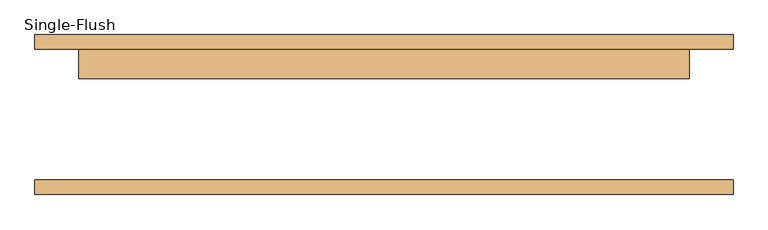
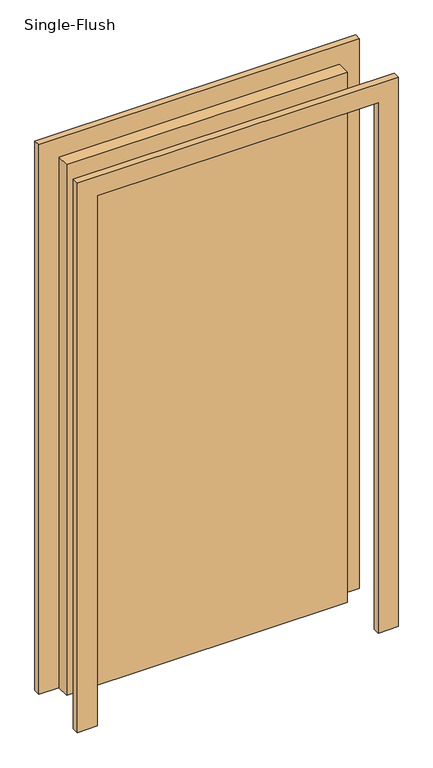
"""IFC4 building model written with IfcOpenShell, lengths in millimetres: door geometry, Single-Flush."""

from ifc_helpers import new_model, si_unit, frame, origin, origin_with_axes, place, context, project, spatial, polyline, outline, extrude, source, transform, mapped, element, save


def single_flush_9d399b00(model_context):
    return source(origin(), model_context, "Body", "SweptSolid", [
        extrude(outline(polyline([(2209.8, -609.6), (0.0, -609.6), (0.0, -533.4), (2133.6, -533.4), (2133.6, 533.4), (0.0, 533.4), (0.0, 609.6), (2209.8, 609.6), (2209.8, -609.6)])), frame((0.0, 114.3, 0.0), z_axis=(0.0, 1.0, 0.0), x_axis=(0.0, 0.0, 1.0)), (0.0, 0.0, 1.0), 25.4),
        extrude(outline(polyline([(2209.8, 609.6), (2209.8, -609.6), (0.0, -609.6), (0.0, -533.4), (2133.6, -533.4), (2133.6, 533.4), (0.0, 533.4), (0.0, 609.6), (2209.8, 609.6)])), frame((0.0, -139.7, 0.0), z_axis=(0.0, 1.0, 0.0), x_axis=(0.0, 0.0, 1.0)), (0.0, 0.0, 1.0), 25.4),
        extrude(outline(polyline([(533.4, 63.5), (-533.4, 63.5), (-533.4, 114.3), (533.4, 114.3), (533.4, 63.5)])), origin_with_axes(), (0.0, 0.0, 1.0), 2133.6),
    ])


if __name__ == "__main__":
    model = new_model("IFC4")
    model_context = context("Model", 3, world=origin())
    ifc_project = project(units=[si_unit("LENGTHUNIT", "METRE", prefix="MILLI")], contexts=[model_context])
    site = spatial("IfcSite", under=ifc_project)
    building = spatial("IfcBuilding", under=site)
    placement = place(None, origin())
    single_flush_shape = single_flush_9d399b00(model_context)
    element("IfcDoor", 1, ObjectType="Single-Flush", at=placement, inside=building, context=model_context, shape_type="MappedRepresentation", body=[
        mapped(single_flush_shape, transform((0.0, 0.0, 0.0), x_axis=(1.0, 0.0, 0.0), y_axis=(0.0, 1.0, 0.0), z_axis=(0.0, 0.0, 1.0))),
    ])
    save(model, "model.ifc")

# Revit data of these elements
# Type "Single-Flush"
#   Type Mark = "8"
#   Construction Type Id = "MDOOR"
#   Assembly Code = "C1020"
#   Analytic Construction = "Metal"
#   Thickness = 0' - 2"
#   Heat Transfer Coefficient (U) = 0.651978 BTU/(h·ft²·°F)
#   Height = 7' - 0"
#   Trim Projection Ext = 0' - 1"
#   Trim Projection Int = 0' - 1"
#   Trim Width = 0' - 3"
#   Width = 3' - 6"
#   Define Thermal Properties by = 1
#   Door Material = Door - Panel
#   Frame Material = Door - Frame
#   Visual Light Transmittance = 0
#   Solar Heat Gain Coefficient = 0
#   Function = (empty or 0)
#   Wall Closure = (empty or 0)
# Element 1 (IfcDoor, "Single-Flush")
#   Materials on its faces: "Door - Frame", "Door - Panel"
# Materials
#   "Door - Panel": class "Wood", colour RGB 210 159 95, transparency 0, Cost = 0
#   "Door - Frame": colour RGB 118 70 51, transparency 0, Cost = 0
